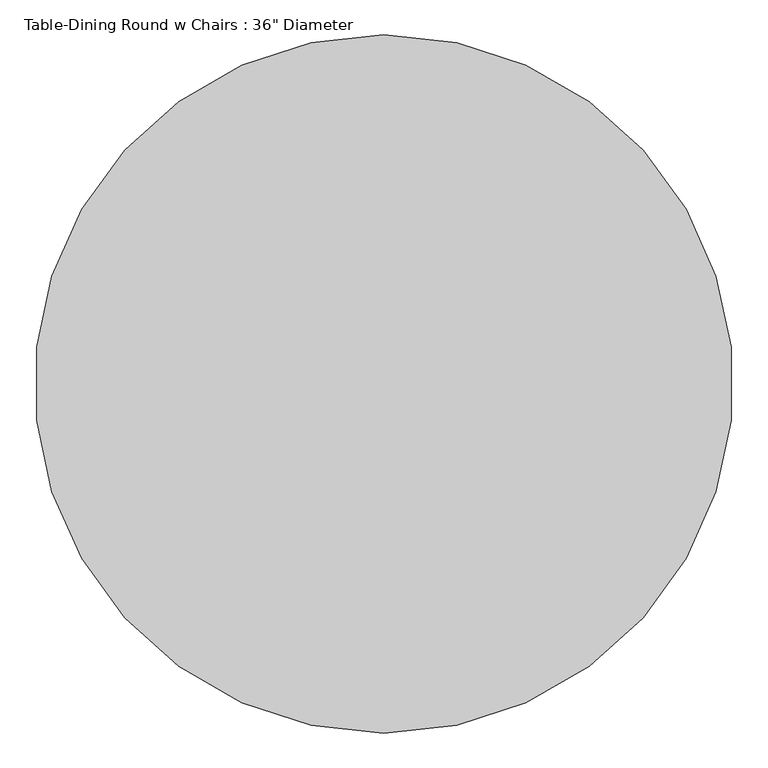
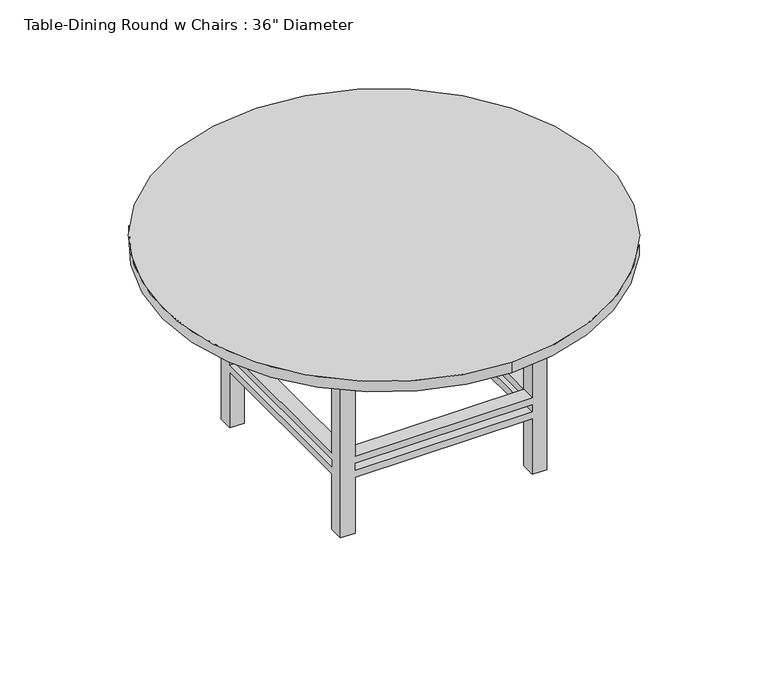
"""IFC4 building model written with IfcOpenShell, lengths in millimetres: furniture geometry."""

from ifc_helpers import new_model, si_unit, point, frame, frame_2d, origin, place, context, project, spatial, polyline, circle_curve, trimmed, segment, composite_curve, outline, extrude, faceted_brep, source, transform, mapped, element, save


def furniture_bbcc68ce(model_context):
    return source(origin(), model_context, "Body", "SolidModel", [
        faceted_brep([(408.4819672, 119.9213115, 279.4), (408.4819672, -489.6786885, 279.4), (459.2819672, -489.6786885, 279.4), (459.2819672, 119.9213115, 279.4), (-201.1180328, -489.6786885, 279.4), (-201.1180328, -540.4786885, 279.4), (408.4819672, -540.4786885, 279.4), (-201.1180328, 119.9213115, 279.4), (-251.9180328, 119.9213115, 279.4), (-251.9180328, -489.6786885, 279.4), (408.4819672, 170.7213115, 279.4), (-201.1180328, 170.7213115, 279.4), (408.4819672, 119.9213115, 254.0), (-201.1180328, 119.9213115, 254.0), (-201.1180328, 170.7213115, 254.0), (408.4819672, 170.7213115, 254.0), (-201.1180328, -489.6786885, 254.0), (-251.9180328, -489.6786885, 254.0), (-251.9180328, 119.9213115, 254.0), (408.4819672, -489.6786885, 254.0), (408.4819672, -540.4786885, 254.0), (-201.1180328, -540.4786885, 254.0), (459.2819672, 119.9213115, 254.0), (459.2819672, -489.6786885, 254.0), (-251.9180328, 170.7213115, 647.7), (-201.1180328, 170.7213115, 647.7), (408.4819672, 170.7213115, 647.7), (459.2819672, 170.7213115, 647.7), (459.2819672, 170.7213115, 0.0), (408.4819672, 170.7213115, 0.0), (408.4819672, 170.7213115, 203.2), (-201.1180328, 170.7213115, 203.2), (-201.1180328, 170.7213115, 0.0), (-251.9180328, 170.7213115, 0.0), (-201.1180328, 170.7213115, 228.6), (408.4819672, 170.7213115, 228.6), (-251.9180328, 119.9213115, 647.7), (-251.9180328, 119.9213115, 0.0), (-251.9180328, 119.9213115, 203.2), (-251.9180328, -489.6786885, 203.2), (-251.9180328, -489.6786885, 0.0), (-251.9180328, -540.4786885, 0.0), (-251.9180328, -540.4786885, 647.7), (-251.9180328, -489.6786885, 647.7), (-251.9180328, -489.6786885, 228.6), (-251.9180328, 119.9213115, 228.6), (459.2819672, -540.4786885, 647.7), (408.4819672, -540.4786885, 647.7), (-201.1180328, -540.4786885, 647.7), (-201.1180328, -540.4786885, 0.0), (-201.1180328, -540.4786885, 203.2), (408.4819672, -540.4786885, 203.2), (408.4819672, -540.4786885, 0.0), (459.2819672, -540.4786885, 0.0), (408.4819672, -540.4786885, 228.6), (-201.1180328, -540.4786885, 228.6), (459.2819672, 119.9213115, 647.7), (459.2819672, -489.6786885, 647.7), (459.2819672, -489.6786885, 0.0), (459.2819672, -489.6786885, 203.2), (459.2819672, 119.9213115, 203.2), (459.2819672, 119.9213115, 0.0), (459.2819672, 119.9213115, 228.6), (459.2819672, -489.6786885, 228.6), (-201.1180328, 119.9213115, 647.7), (408.4819672, -489.6786885, 647.7), (408.4819672, 119.9213115, 647.7), (-201.1180328, -489.6786885, 647.7), (408.4819672, 119.9213115, 0.0), (-201.1180328, -489.6786885, 0.0), (-201.1180328, 119.9213115, 0.0), (408.4819672, -489.6786885, 0.0), (-201.1180328, 119.9213115, 228.6), (-201.1180328, 119.9213115, 203.2), (408.4819672, 119.9213115, 228.6), (408.4819672, 119.9213115, 203.2), (408.4819672, -489.6786885, 228.6), (408.4819672, -489.6786885, 203.2), (-201.1180328, -489.6786885, 228.6), (-201.1180328, -489.6786885, 203.2)], [[[0, 1, 2, 3]], [[1, 4, 5, 6]], [[4, 7, 8, 9]], [[7, 0, 10, 11]], [[12, 13, 14, 15]], [[13, 16, 17, 18]], [[16, 19, 20, 21]], [[19, 12, 22, 23]], [[24, 25, 11, 10, 26, 27, 28, 29, 30, 31, 32, 33], [14, 34, 35, 15]], [[36, 24, 33, 37, 38, 39, 40, 41, 42, 43, 9, 8], [17, 44, 45, 18]], [[46, 47, 6, 5, 48, 42, 41, 49, 50, 51, 52, 53], [20, 54, 55, 21]], [[28, 27, 56, 3, 2, 57, 46, 53, 58, 59, 60, 61], [22, 62, 63, 23]], [[1, 0, 12, 19]], [[4, 1, 19, 16]], [[7, 4, 16, 13]], [[0, 7, 13, 12]], [[25, 24, 36, 64]], [[47, 46, 57, 65]], [[26, 66, 56, 27]], [[48, 67, 43, 42]], [[29, 28, 61, 68]], [[49, 41, 40, 69]], [[32, 70, 37, 33]], [[52, 71, 58, 53]], [[13, 18, 45, 72]], [[64, 36, 8, 7]], [[37, 70, 73, 38]], [[14, 13, 72, 34]], [[25, 64, 7, 11]], [[70, 32, 31, 73]], [[12, 15, 35, 74]], [[66, 26, 10, 0]], [[29, 68, 75, 30]], [[22, 12, 74, 62]], [[56, 66, 0, 3]], [[68, 61, 60, 75]], [[19, 23, 63, 76]], [[65, 57, 2, 1]], [[58, 71, 77, 59]], [[20, 19, 76, 54]], [[47, 65, 1, 6]], [[71, 52, 51, 77]], [[16, 21, 55, 78]], [[67, 48, 5, 4]], [[49, 69, 79, 50]], [[17, 16, 78, 44]], [[43, 67, 4, 9]], [[69, 40, 39, 79]], [[74, 76, 63, 62]], [[76, 78, 55, 54]], [[78, 72, 45, 44]], [[72, 74, 35, 34]], [[75, 73, 31, 30]], [[73, 79, 39, 38]], [[79, 77, 51, 50]], [[77, 75, 60, 59]], [[76, 74, 75, 77]], [[78, 76, 77, 79]], [[72, 78, 79, 73]], [[74, 72, 73, 75]]]),
        extrude(outline(polyline([(484.6819672, 196.1213115), (484.6819672, -565.8786885), (-277.3180328, -565.8786885), (-277.3180328, 196.1213115), (484.6819672, 196.1213115)]), holes=[polyline([(459.2819672, 170.7213115), (-251.9180328, 170.7213115), (-251.9180328, -540.4786885), (459.2819672, -540.4786885), (459.2819672, 170.7213115)])]), frame((0.0, 0.0, 647.7), z_axis=(0.0, 0.0, 1.0), x_axis=(1.0, 0.0, 0.0)), (0.0, 0.0, 1.0), 76.2),
        extrude(outline(composite_curve([segment(trimmed(circle_curve(frame_2d((103.6819672, -184.8786885)), 762.0), [point((103.6819672, -946.8786885))], [point((103.6819672, 577.1213115))], False, "CARTESIAN"), True, "CONTINUOUS"), segment(trimmed(circle_curve(frame_2d((103.6819672, -184.8786885)), 762.0), [point((103.6819672, 577.1213115))], [point((103.6819672, -946.8786885))], False, "CARTESIAN"), True, "CONTINUOUS")], self_intersect=False)), frame((0.0, 0.0, 723.9), z_axis=(0.0, 0.0, 1.0), x_axis=(1.0, 0.0, 0.0)), (0.0, 0.0, 1.0), 38.1),
    ])


if __name__ == "__main__":
    model = new_model("IFC4")
    model_context = context("Model", 3, world=origin())
    ifc_project = project(units=[si_unit("LENGTHUNIT", "METRE", prefix="MILLI")], contexts=[model_context])
    site = spatial("IfcSite", under=ifc_project)
    building = spatial("IfcBuilding", under=site)
    placement = place(None, origin())
    furniture_shape = furniture_bbcc68ce(model_context)
    element("IfcFurniture", 1, ObjectType="Table-Dining Round w Chairs : 36\" Diameter", at=placement, inside=building, context=model_context, shape_type="MappedRepresentation", body=[
        mapped(furniture_shape, transform((0.0, 0.0, 0.0), x_axis=(1.0, 0.0, 0.0), y_axis=(0.0, 1.0, 0.0), z_axis=(0.0, 0.0, 1.0))),
    ])
    save(model, "model.ifc")

# Revit data of these elements
# Type "Table-Dining Round w Chairs : 36\" Diameter"
#   Assembly Code = "E2020200"
#   Radius = 2' - 6"
#   Diameter = 5' - 0"
#   Height = 2' - 6"
#   Chairs = 6
#   Base Material = Pine
#   Top Material = Laminate, Linen, Matte
#   Default Elevation = 0
# Element 1 (IfcFurniture, "Table-Dining Round w Chairs : 36\" Diameter")
#   Materials on its faces: "Pine", "Laminate, Linen, Matte"
# Materials
#   "Pine": class "Wood", colour RGB 223 192 134, transparency 0, Description = "Pinus Echinata", Cost = 0
#   "Laminate, Linen, Matte": class "Plastic", colour RGB 249 239 230, transparency 0, Description = "Plastic Laminate - Linen, Matte", Cost = 0
